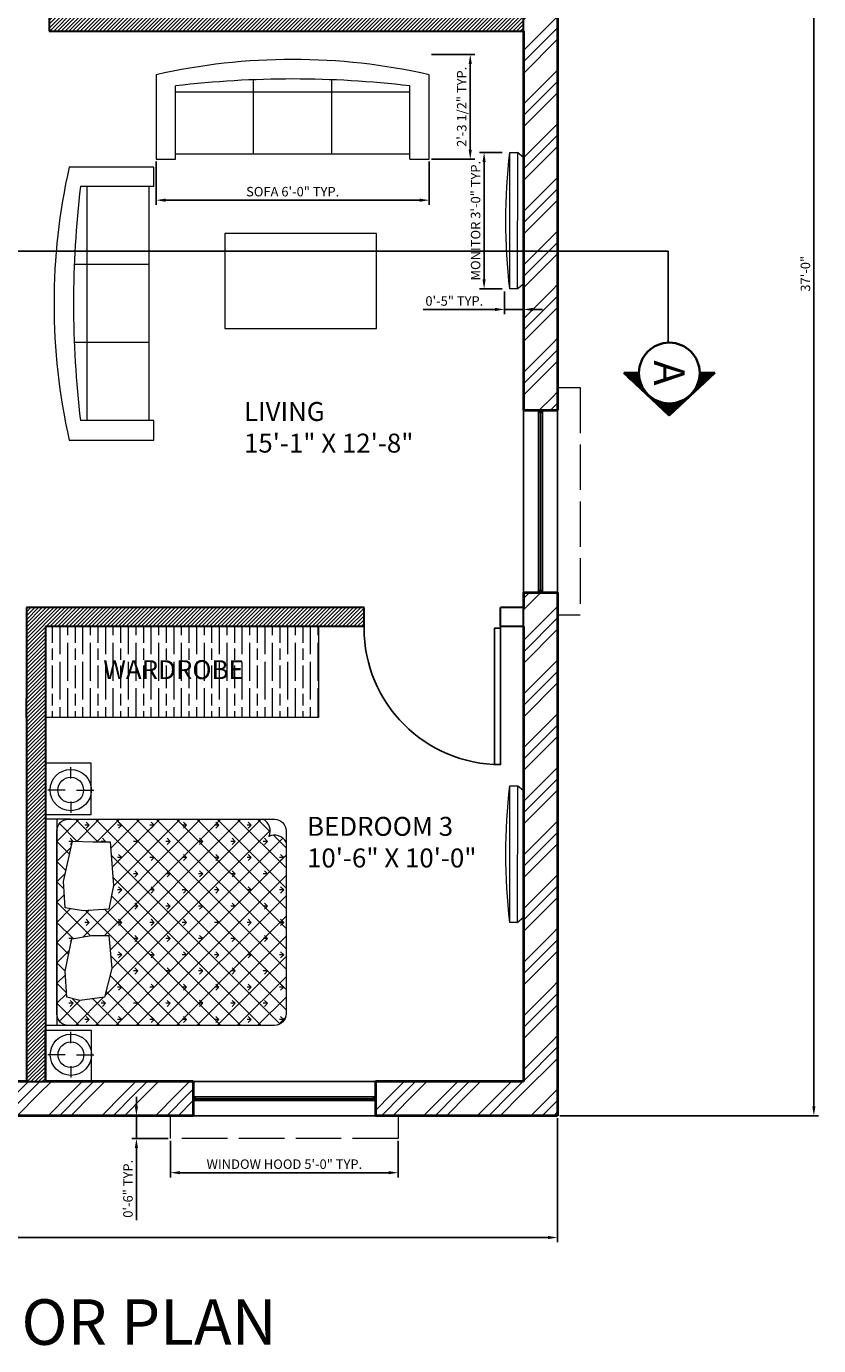
# Model space of a CAD drawing. Units: inches. Extents: x 2443635 to 2446153, y 1826255 to 1827341.
# Tile 4 of 16: x 2443891 to 2444100, y 1826801 to 1827149. Entities that reach past the tile are written whole.
import ezdxf
from ezdxf.enums import TextEntityAlignment as Align

# ---------------------------------------------------------------- set-up
doc = ezdxf.new("R2010")
doc.units = ezdxf.units.IN
doc.linetypes.add('ACAD_ISO02W100', pattern=[15, 12, -3])
for name, color, linetype, lineweight in [('A-ANNO-SYMB', 4, 'Continuous', 25), ('A-DIMS', 1, 'Continuous', 18), ('A-DOOR', 2, 'Continuous', 25), ('A-EQPM', 8, 'Continuous', 18), ('A-FLOR-CASE', 8, 'Continuous', 18), ('A-FLOR-CASE-PATT', 252, 'Continuous', 13), ('A-FURN', 6, 'Continuous', 18), ('A-ROOM', 4, 'Continuous', 18), ('A-SECT', 7, 'Continuous', 35), ('A-TEXT', 4, 'Continuous', 25), ('A-WALL-EXT', 7, 'Continuous', 40), ('A-WALL-INT', 9, 'Continuous', 30), ('A-WALL-OVHD', 7, 'ACAD_ISO02W100', 18), ('A-WALL-PATT', 8, 'Continuous', 13), ('A-WINDOW', 4, 'Continuous', 25)]:
    doc.layers.add(name, color=color, linetype=linetype, lineweight=lineweight)
doc.styles.add('KH-TRUC', font='txt', dxfattribs={"height": 200})
doc.styles.get("Standard").update_dxf_attribs({"font": 'arial.ttf'})
doc.dimstyles.new('ISO-25', dxfattribs={"dimtxt": 2.5, "dimasz": 2.5, "dimexe": 1.25, "dimexo": 0.625, "dimtad": 1, "dimlunit": 4, "dimtxsty": 'Standard', "dimcen": 2.5, "dimadec": 0, "dimazin": 0, "dimtfac": 1, "dimtmove": 0, "dimatfit": 3, "dimfxl": 1, "dimarcsym": 0})

# ---------------------------------------------------------------- blocks, each defined once
blk = doc.blocks.new('*U3')
for p, q in [((0, 0), (0, -6)), ((-40, 0), (-40, -6))]:
    blk.add_line(p, q)
blk.add_lwpolyline([(0, 0), (0, 40), (-1.75, 40), (-1.75, 0)], close=True)
blk.add_arc((0, 0), 40, 90, 180)
blk = doc.blocks.new('*X6')
at = {"color": 0}
for p, q in [((0, 0), (0, 0)), ((-707, -141), (-734, -115)), ((-707, -141), (-707, -104)), ((-707, -141), (-681, -115)), ((-566, 0), (-566, 0)), ((-566, 0), (-566, 0)), ((-283, 0), (-283, 0)), ((-283, 0), (-283, 0)), ((-156, -126), (-168, -115)), ((-141, -141), (-141, -104)), ((-141, -141), (-115, -115)), ((120, -120), (115, -115)), ((283, 0), (283, 0)), ((566, 0), (566, 0)), ((699, -134), (681, -115)), ((707, -135), (707, -104)), ((710, -139), (734, -115)), ((-141, -141), (-142, -140)), ((-849, -283), (-875, -256)), ((-849, -283), (-849, -245)), ((-849, -283), (-822, -256)), ((0, -283), (-27, -256)), ((0, -283), (0, -245)), ((0, -283), (27, -256)), ((849, -283), (822, -256)), ((849, -283), (849, -245)), ((849, -283), (875, -256)), ((-707, -424), (-734, -398)), ((-707, -424), (-707, -387)), ((-707, -424), (-681, -398)), ((-116, -399), (-115, -398)), ((707, -424), (703, -420)), ((707, -424), (707, -387)), ((707, -424), (734, -398)), ((-849, -566), (-875, -539)), ((-849, -566), (-849, -528)), ((-849, -566), (-822, -539)), ((-566, -566), (-592, -539)), ((-566, -566), (-566, -528)), ((-566, -566), (-539, -539)), ((-283, -566), (-309, -539)), ((-283, -566), (-283, -528)), ((-283, -566), (-256, -539)), ((0, -566), (-27, -539)), ((0, -566), (0, -528)), ((0, -566), (27, -539)), ((283, -566), (256, -539)), ((283, -566), (283, -528)), ((283, -566), (309, -539)), ((566, -566), (539, -539)), ((566, -566), (566, -528)), ((566, -566), (592, -539)), ((849, -566), (822, -539)), ((849, -566), (849, -528)), ((849, -566), (875, -539)), ((-707, -707), (-734, -681)), ((-707, -707), (-707, -670)), ((-707, -707), (-681, -681)), ((-424, -707), (-451, -681)), ((-424, -707), (-424, -670)), ((-424, -707), (-398, -681)), ((-141, -707), (-168, -681)), ((-141, -707), (-141, -670)), ((-141, -707), (-115, -681)), ((141, -707), (115, -681)), ((141, -707), (141, -670)), ((141, -707), (168, -681)), ((424, -707), (398, -681)), ((424, -707), (424, -670)), ((424, -707), (451, -681)), ((707, -707), (681, -681)), ((707, -707), (707, -670)), ((707, -707), (734, -681)), ((-849, -849), (-875, -822)), ((-849, -849), (-849, -811)), ((-849, -849), (-822, -822)), ((-566, -849), (-592, -822)), ((-566, -849), (-566, -811)), ((-566, -849), (-539, -822)), ((-283, -849), (-309, -822)), ((-283, -849), (-283, -811)), ((-283, -849), (-256, -822)), ((0, -849), (-27, -822)), ((0, -849), (0, -811)), ((0, -849), (27, -822)), ((283, -849), (256, -822)), ((283, -849), (283, -811)), ((283, -849), (309, -822)), ((566, -849), (539, -822)), ((566, -849), (566, -811)), ((566, -849), (592, -822)), ((849, -849), (822, -822)), ((849, -849), (849, -811)), ((849, -849), (875, -822)), ((-707, -990), (-734, -963)), ((-707, -990), (-707, -952)), ((-707, -990), (-681, -963)), ((-424, -990), (-451, -963)), ((-424, -990), (-424, -952)), ((-424, -990), (-398, -963)), ((-141, -990), (-168, -963)), ((-141, -990), (-141, -952)), ((-141, -990), (-115, -963)), ((141, -990), (115, -963)), ((141, -990), (141, -952)), ((141, -990), (168, -963)), ((424, -990), (398, -963)), ((424, -990), (424, -952)), ((424, -990), (451, -963)), ((707, -990), (681, -963)), ((707, -990), (707, -952)), ((707, -990), (734, -963)), ((-849, -1131), (-875, -1105)), ((-849, -1131), (-849, -1094)), ((-849, -1131), (-822, -1105)), ((-566, -1131), (-592, -1105)), ((-566, -1131), (-566, -1094)), ((-566, -1131), (-539, -1105)), ((-283, -1131), (-309, -1105)), ((-283, -1131), (-283, -1094)), ((-283, -1131), (-256, -1105)), ((0, -1131), (-27, -1105)), ((0, -1131), (0, -1094)), ((0, -1131), (27, -1105)), ((283, -1131), (256, -1105)), ((283, -1131), (283, -1094)), ((283, -1131), (309, -1105)), ((566, -1131), (539, -1105)), ((566, -1131), (566, -1094)), ((566, -1131), (592, -1105)), ((849, -1131), (822, -1105)), ((849, -1131), (849, -1094)), ((849, -1131), (875, -1105)), ((-707, -1273), (-734, -1246)), ((-707, -1273), (-707, -1235)), ((-707, -1273), (-681, -1246)), ((-424, -1273), (-451, -1246)), ((-424, -1273), (-424, -1235)), ((-424, -1273), (-398, -1246)), ((-141, -1273), (-168, -1246)), ((-141, -1273), (-141, -1235)), ((-141, -1273), (-115, -1246)), ((141, -1273), (115, -1246)), ((141, -1273), (141, -1235)), ((141, -1273), (168, -1246)), ((424, -1273), (398, -1246)), ((424, -1273), (424, -1235)), ((424, -1273), (451, -1246)), ((707, -1273), (681, -1246)), ((707, -1273), (707, -1235)), ((707, -1273), (734, -1246)), ((-849, -1414), (-849, -1377)), ((-566, -1414), (-566, -1377)), ((-283, -1414), (-283, -1377)), ((0, -1414), (0, -1377)), ((283, -1414), (283, -1377)), ((566, -1414), (566, -1377)), ((849, -1414), (849, -1377)), ((-849, -1414), (-875, -1388)), ((-849, -1414), (-822, -1388)), ((-566, -1414), (-592, -1388)), ((-566, -1414), (-539, -1388)), ((-283, -1414), (-309, -1388)), ((-283, -1414), (-256, -1388)), ((0, -1414), (-27, -1388)), ((0, -1414), (27, -1388)), ((283, -1414), (256, -1388)), ((283, -1414), (309, -1388)), ((566, -1414), (539, -1388)), ((566, -1414), (592, -1388)), ((849, -1414), (822, -1388)), ((849, -1414), (875, -1388)), ((-707, -1556), (-734, -1529)), ((-707, -1556), (-707, -1518)), ((-707, -1556), (-681, -1529)), ((-424, -1556), (-451, -1529)), ((-424, -1556), (-424, -1518)), ((-424, -1556), (-398, -1529)), ((-141, -1556), (-168, -1529)), ((-141, -1556), (-141, -1518)), ((-141, -1556), (-115, -1529)), ((141, -1556), (115, -1529)), ((141, -1556), (141, -1518)), ((141, -1556), (168, -1529)), ((424, -1556), (398, -1529)), ((424, -1556), (424, -1518)), ((424, -1556), (451, -1529)), ((707, -1556), (681, -1529)), ((707, -1556), (707, -1518)), ((707, -1556), (734, -1529)), ((-849, -1697), (-875, -1671)), ((-849, -1697), (-849, -1660)), ((-849, -1697), (-822, -1671)), ((-566, -1697), (-592, -1671)), ((-566, -1697), (-566, -1660)), ((-566, -1697), (-539, -1671)), ((-283, -1697), (-309, -1671)), ((-283, -1697), (-283, -1660)), ((-283, -1697), (-256, -1671)), ((0, -1697), (-27, -1671)), ((0, -1697), (0, -1660)), ((0, -1697), (27, -1671)), ((283, -1697), (256, -1671)), ((283, -1697), (283, -1660)), ((283, -1697), (309, -1671)), ((566, -1697), (539, -1671)), ((566, -1697), (566, -1660)), ((566, -1697), (592, -1671)), ((849, -1697), (822, -1671)), ((849, -1697), (849, -1660)), ((849, -1697), (875, -1671)), ((-707, -1838), (-734, -1812)), ((-707, -1838), (-707, -1801)), ((-707, -1838), (-681, -1812)), ((-424, -1838), (-451, -1812)), ((-424, -1838), (-424, -1801)), ((-424, -1838), (-398, -1812)), ((-141, -1838), (-168, -1812)), ((-141, -1838), (-141, -1801)), ((-141, -1838), (-115, -1812)), ((141, -1838), (115, -1812)), ((141, -1838), (141, -1801)), ((141, -1838), (168, -1812)), ((424, -1838), (398, -1812)), ((424, -1838), (424, -1801)), ((424, -1838), (451, -1812)), ((707, -1838), (681, -1812)), ((707, -1838), (707, -1801)), ((707, -1838), (734, -1812)), ((-849, -1980), (-875, -1953)), ((-849, -1980), (-849, -1942)), ((-849, -1980), (-822, -1953)), ((-566, -1980), (-592, -1953)), ((-566, -1980), (-566, -1942)), ((-566, -1980), (-539, -1953)), ((-283, -1980), (-309, -1953)), ((-283, -1980), (-283, -1942)), ((-283, -1980), (-256, -1953)), ((0, -1980), (-27, -1953)), ((0, -1980), (0, -1942)), ((0, -1980), (27, -1953)), ((283, -1980), (256, -1953)), ((283, -1980), (283, -1942)), ((283, -1980), (309, -1953)), ((566, -1980), (539, -1953)), ((566, -1980), (566, -1942)), ((566, -1980), (592, -1953))]:
    blk.add_line(p, q, dxfattribs=at)
blk = doc.blocks.new('*X5')
at = {"color": 0}
for p, q in [((-900, -193), (-707, 0)), ((-623, -84), (-707, 0)), ((-614, -83), (-530, 0)), ((-457, -74), (-530, 0)), ((-425, -72), (-354, 0)), ((-245, -108), (-354, 0)), ((-278, -101), (-177, 0)), ((103, -280), (-177, 0)), ((-142, -142), (0, 0)), ((-117, -294), (177, 0)), ((120, -120), (0, 0)), ((241, -64), (177, 0)), ((292, -61), (354, 0)), ((426, -72), (354, 0)), ((452, -78), (530, 0)), ((654, -123), (530, 0)), ((596, -111), (707, 0)), ((900, -193), (707, 0)), ((-683, -201), (-862, -22)), ((708, -175), (862, -22)), ((-900, -370), (-667, -137)), ((-656, -405), (-900, -161)), ((900, -1254), (-128, -225)), ((703, -358), (900, -161)), ((900, -370), (708, -178)), ((-900, -1254), (101, -252)), ((-900, -546), (-668, -314)), ((735, -1973), (-900, -337)), ((-763, -2000), (900, -337)), ((-900, -1430), (112, -418)), ((-900, -723), (-605, -429)), ((801, -1862), (-641, -419)), ((900, -1430), (-116, -415)), ((900, -546), (703, -349)), ((-900, -900), (-465, -465)), ((-900, -1077), (-293, -470)), ((-900, -1607), (231, -476)), ((-900, -1784), (394, -489)), ((586, -2000), (-900, -514)), ((-888, -1948), (586, -475)), ((-586, -2000), (900, -514)), ((900, -1784), (-404, -480)), ((900, -1607), (-243, -465)), ((900, -1077), (317, -494)), ((900, -900), (483, -483)), ((900, -723), (647, -470)), ((409, -2000), (-900, -691)), ((-409, -2000), (900, -691)), ((232, -2000), (-900, -868)), ((-232, -2000), (900, -868)), ((55, -2000), (-900, -1045)), ((-55, -2000), (900, -1045)), ((-121, -2000), (-900, -1221)), ((121, -2000), (900, -1221)), ((-298, -2000), (-900, -1398)), ((298, -2000), (900, -1398)), ((-475, -2000), (-900, -1575)), ((475, -2000), (900, -1575)), ((-652, -2000), (-900, -1752)), ((790, -1861), (900, -1752)), ((-835, -1994), (-894, -1935)), ((652, -2000), (761, -1890))]:
    blk.add_line(p, q, dxfattribs=at)
blk = doc.blocks.new('A$C190D2546')
at = {"layer": 'A-FURN'}
for p, q in [((285, 1928), (285, 2078)), ((541, 2100), (2341, 2100)), ((541, 1881), (541, 2100)), ((2341, 1881), (2341, 2100)), ((2596, 1929), (2596, 2079)), ((2341, 2000), (541, 2000)), ((185, 1878), (85, 1878)), ((385, 1878), (485, 1878)), ((2496, 1879), (2396, 1879)), ((2696, 1879), (2796, 1879)), ((285, 1828), (285, 1678)), ((2596, 1829), (2596, 1679))]:
    blk.add_line(p, q, dxfattribs=at)
for points in [[(500, 2101), (500, 1701), (50, 1701), (50, 2101)], [(2382, 2101), (2382, 1701), (2832, 1701), (2832, 2101)], [(787, 1584), (758, 1799), (787, 1914), (1016, 1928), (1296, 1871), (1325, 1699), (1325, 1548), (1038, 1519)], [(1555, 1548), (1541, 1771), (1569, 1928), (1799, 1943), (2151, 1864), (2144, 1685), (2144, 1534), (1763, 1505)]]:
    blk.add_lwpolyline(points, close=True, dxfattribs=at)
blk.add_lwpolyline([(641, 2000), (2241, 2000, -0.414214), (2341, 1900), (2341, 100, -0.414214), (2241, 0), (641, 0, -0.414214), (541, 100), (541, 1900, -0.414214)], format="xyb", close=True, dxfattribs=at)
for centre, radius in [((285, 1878), 180), ((285, 1878), 112), ((2596, 1879), 180), ((2596, 1879), 112)]:
    blk.add_circle(centre, radius, dxfattribs=at)
for centre, start, end in [((2091, 100), 296.5651, 26.5651), ((2241, 250), 243.4349, 333.4349)]:
    blk.add_arc(centre, 112, start, end, dxfattribs=at)
for name in ['*X5', '*X6']:
    blk.add_blockref(name, (1441, 2000), dxfattribs=at)
blk = doc.blocks.new('LCD Monitor Pln')
at = {"layer": 'A-FURN'}
for p, q in [((5656.37, -10564.55), (5660.02, -10561.47)), ((5656.37, -10564.55), (5656.4, -10641.11)), ((5660.02, -10561.47), (5660.05, -10644.19)), ((5664.53, -10561.47), (5660.02, -10561.47)), ((5664.56, -10644.19), (5664.53, -10561.47)), ((5660.05, -10644.19), (5656.4, -10641.11)), ((5660.05, -10644.19), (5664.56, -10644.19))]:
    blk.add_line(p, q, dxfattribs=at)
blk.add_arc((5310.21, -10602.95), 356.75, 353.36301, 6.67799, dxfattribs=at)
blk = doc.blocks.new('*X15')
at = {"color": 0}
for p, q in [((19.68, 20.47), (19.71, 20.51)), ((19.68, 20.38), (19.76, 20.46)), ((19.68, 20.29), (19.8, 20.42)), ((19.68, 20.21), (19.84, 20.37)), ((19.68, 20.12), (19.88, 20.33)), ((19.68, 20.03), (19.93, 20.28)), ((19.68, 19.94), (19.97, 20.23)), ((19.68, 19.85), (20.01, 20.19)), ((19.68, 19.76), (20.05, 20.14)), ((19.68, 19.68), (20.1, 20.1)), ((19.68, 19.59), (20.14, 20.05)), ((19.68, 19.5), (20.18, 20.01)), ((19.68, 19.41), (20.22, 19.96)), ((19.68, 19.32), (20.27, 19.91)), ((19.68, 19.23), (20.31, 19.87)), ((19.68, 19.15), (20.35, 19.82)), ((19.68, 19.06), (20.4, 19.78)), ((19.68, 18.97), (20.44, 19.73)), ((19.68, 18.88), (20.48, 19.69)), ((19.68, 18.79), (20.52, 19.64)), ((19.68, 18.7), (20.57, 19.59)), ((19.68, 18.62), (20.61, 19.55)), ((19.68, 18.53), (20.65, 19.5)), ((19.68, 18.44), (20.69, 19.46)), ((19.68, 18.35), (20.74, 19.41)), ((19.68, 18.26), (20.78, 19.37)), ((19.68, 18.17), (20.82, 19.32)), ((19.68, 18.08), (20.86, 19.27)), ((19.73, 18.05), (20.91, 19.23)), ((19.81, 18.05), (20.95, 19.18)), ((19.9, 18.04), (20.99, 19.14)), ((19.98, 18.04), (21.04, 19.09)), ((20.06, 18.03), (21.08, 19.05)), ((20.15, 18.03), (21.12, 19)), ((20.23, 18.02), (21.16, 18.95)), ((20.31, 18.01), (21.21, 18.91)), ((20.38, 18), (21.25, 18.86)), ((20.46, 17.99), (21.29, 18.82)), ((20.54, 17.97), (21.33, 18.77)), ((20.61, 17.96), (21.38, 18.73)), ((20.68, 17.94), (21.42, 18.68)), ((20.76, 17.93), (21.46, 18.63)), ((20.83, 17.91), (21.5, 18.59)), ((20.9, 17.9), (21.55, 18.54)), ((20.97, 17.88), (21.59, 18.5)), ((21.04, 17.86), (21.63, 18.45)), ((21.11, 17.84), (21.68, 18.41)), ((21.18, 17.82), (21.72, 18.36)), ((21.24, 17.8), (21.76, 18.31)), ((21.31, 17.77), (21.8, 18.27)), ((21.37, 17.75), (21.85, 18.22)), ((21.44, 17.73), (21.89, 18.18)), ((21.5, 17.7), (21.93, 18.13)), ((21.57, 17.68), (21.97, 18.08)), ((21.63, 17.65), (22.02, 18.04)), ((21.69, 17.62), (22.06, 17.99)), ((21.75, 17.6), (22.1, 17.95)), ((21.81, 17.57), (22.14, 17.9)), ((21.87, 17.54), (22.19, 17.86)), ((21.93, 17.51), (22.23, 17.81)), ((21.99, 17.48), (22.27, 17.76)), ((22.05, 17.45), (22.32, 17.72)), ((22.1, 17.42), (22.36, 17.67)), ((22.16, 17.39), (22.4, 17.63)), ((22.22, 17.35), (22.44, 17.58)), ((22.27, 17.32), (22.49, 17.54)), ((22.33, 17.29), (22.53, 17.49)), ((22.38, 17.25), (22.57, 17.44)), ((22.43, 17.22), (22.61, 17.4)), ((22.49, 17.18), (22.66, 17.35)), ((22.54, 17.15), (22.7, 17.31)), ((22.59, 17.11), (22.74, 17.26)), ((22.64, 17.07), (22.78, 17.22)), ((22.69, 17.04), (22.83, 17.17)), ((22.74, 17), (22.87, 17.12)), ((22.79, 16.96), (22.91, 17.08)), ((22.84, 16.92), (22.96, 17.03)), ((22.89, 16.88), (23, 16.99)), ((22.94, 16.84), (23.04, 16.94)), ((22.98, 16.8), (23.08, 16.9)), ((23.03, 16.75), (23.13, 16.85)), ((23.08, 16.71), (23.17, 16.8)), ((23.12, 16.67), (23.21, 16.76)), ((23.17, 16.63), (23.25, 16.71)), ((23.21, 16.58), (23.3, 16.67)), ((23.26, 16.54), (23.34, 16.62)), ((23.3, 16.49), (23.38, 16.58)), ((23.34, 16.45), (23.42, 16.53)), ((23.38, 16.4), (23.47, 16.48)), ((23.43, 16.35), (23.51, 16.44)), ((23.47, 16.31), (23.55, 16.39)), ((23.51, 16.26), (23.6, 16.35)), ((23.55, 16.21), (23.64, 16.3)), ((23.59, 16.16), (23.68, 16.26)), ((23.63, 16.11), (23.72, 16.21)), ((23.66, 16.06), (23.77, 16.16)), ((23.7, 16.01), (23.81, 16.12)), ((23.74, 15.96), (23.85, 16.07)), ((23.78, 15.91), (23.89, 16.03)), ((23.81, 15.86), (23.94, 15.98)), ((23.85, 15.8), (23.98, 15.94)), ((23.88, 15.75), (24.02, 15.89)), ((23.92, 15.7), (24.06, 15.84)), ((23.95, 15.64), (24.11, 15.8)), ((23.98, 15.59), (24.15, 15.75)), ((24.02, 15.53), (24.19, 15.71)), ((24.05, 15.47), (24.24, 15.66)), ((24.08, 15.42), (24.28, 15.62)), ((24.11, 15.36), (24.32, 15.57)), ((24.14, 15.3), (24.36, 15.52)), ((24.17, 15.24), (24.41, 15.48)), ((24.2, 15.18), (24.45, 15.43)), ((24.23, 15.12), (24.49, 15.39)), ((24.25, 15.06), (24.53, 15.34)), ((24.28, 15), (24.58, 15.3)), ((24.31, 14.94), (24.62, 15.25)), ((23.72, 10.11), (26.67, 13.06)), ((23.91, 10.38), (26.63, 13.1)), ((24.04, 10.6), (26.58, 13.15)), ((24.14, 10.79), (26.54, 13.19)), ((24.22, 10.96), (26.5, 13.24)), ((24.29, 11.12), (26.45, 13.28)), ((24.33, 14.87), (24.66, 15.2)), ((24.35, 11.27), (26.41, 13.33)), ((24.36, 14.81), (24.7, 15.16)), ((24.38, 14.74), (24.75, 15.11)), ((24.4, 14.68), (24.79, 15.07)), ((24.4, 11.41), (26.37, 13.38)), ((24.42, 14.61), (24.83, 15.02)), ((24.44, 11.54), (26.33, 13.42)), ((24.45, 14.55), (24.88, 14.98)), ((24.47, 14.48), (24.92, 14.93)), ((24.48, 11.66), (26.28, 13.47)), ((24.49, 14.41), (24.96, 14.88)), ((24.51, 14.34), (25, 14.84)), ((24.51, 11.79), (26.24, 13.51)), ((24.52, 14.27), (25.05, 14.79)), ((24.54, 14.2), (25.09, 14.75)), ((24.54, 11.9), (26.2, 13.56)), ((24.56, 14.13), (25.13, 14.7)), ((24.57, 14.06), (25.17, 14.66)), ((24.57, 12.02), (26.16, 13.6)), ((24.59, 13.98), (25.22, 14.61)), ((24.59, 12.13), (26.11, 13.65)), ((24.6, 13.91), (25.26, 14.56)), ((24.61, 13.83), (25.3, 14.52)), ((24.61, 12.24), (26.07, 13.7)), ((24.63, 13.75), (25.35, 14.47)), ((24.63, 12.34), (26.03, 13.74)), ((24.64, 13.68), (25.39, 14.43)), ((24.64, 12.44), (25.99, 13.79)), ((24.65, 13.6), (25.43, 14.38)), ((24.65, 13.52), (25.47, 14.34)), ((24.65, 12.54), (25.94, 13.83)), ((24.66, 13.44), (25.52, 14.29)), ((24.66, 12.64), (25.9, 13.88)), ((24.67, 13.35), (25.56, 14.24)), ((24.67, 13.27), (25.6, 14.2)), ((24.67, 13.18), (25.64, 14.15)), ((24.67, 12.92), (25.77, 14.02)), ((24.67, 12.83), (25.81, 13.97)), ((24.67, 12.73), (25.86, 13.92)), ((24.68, 13.1), (25.69, 14.11)), ((24.68, 13.01), (25.73, 14.06)), ((19.68, 5.98), (25.68, 11.98)), ((19.68, 5.89), (24.44, 10.65)), ((19.68, 5.8), (23.2, 9.32)), ((19.68, 6.06), (22.61, 9)), ((19.68, 6.15), (22.34, 8.81)), ((19.68, 6.24), (22.12, 8.69)), ((19.68, 6.33), (21.93, 8.58)), ((19.68, 6.42), (21.76, 8.5)), ((19.68, 6.51), (21.6, 8.43)), ((19.68, 6.59), (21.46, 8.37)), ((19.68, 6.68), (21.32, 8.32)), ((19.68, 6.77), (21.19, 8.28)), ((19.68, 6.86), (21.06, 8.24)), ((19.68, 6.95), (20.94, 8.21)), ((19.68, 7.04), (20.82, 8.18)), ((19.68, 7.12), (20.71, 8.15)), ((19.68, 7.21), (20.6, 8.13)), ((19.68, 7.3), (20.49, 8.11)), ((19.68, 7.39), (20.38, 8.1)), ((19.68, 7.48), (20.28, 8.08)), ((19.68, 7.57), (20.18, 8.07)), ((19.68, 7.74), (19.99, 8.06)), ((19.68, 7.66), (20.08, 8.06)), ((19.68, 8.01), (19.71, 8.05)), ((19.68, 7.92), (19.8, 8.05)), ((19.68, 7.83), (19.9, 8.05)), ((19.68, 5.71), (21.96, 8)), ((19.68, 5.62), (20.73, 6.67))]:
    blk.add_line(p, q, dxfattribs=at)
blk = doc.blocks.new('A$C0BB45C51')
at = {"layer": 'A-SECT'}
for p, q in [((12.86, 15), (19.86, 7.5)), ((12.86, 12.5), (12.86, 15)), ((12.86, 0), (19.86, 7.5)), ((12.86, 2.5), (12.86, 0))]:
    blk.add_line(p, q, dxfattribs=at)
blk.add_circle((12.86, 7.5), 5, dxfattribs=at)
blk.add_blockref('*X15', (-6.82, -5.55), dxfattribs=at)
at = {"layer": 'A-SECT', "style": 'KH-TRUC'}
blk.add_attdef('KH-MC', text='', height=5, dxfattribs=at).set_placement((12.86, 7.5), align=Align.MIDDLE_CENTER)
blk = doc.blocks.new('SOFA-3-SEAT')
at = {"transparency": 33554687}
for p, q in [((0, 22.29), (0, 0)), ((25.71, 1.34), (25.71, 20.94)), ((46.29, 1.34), (46.29, 20.94)), ((72, 0), (72, 22.29)), ((5.14, 0), (5.14, 19.31)), ((66.86, 17.67), (5.14, 17.67)), ((66.86, 0), (66.86, 19.31)), ((0, 0), (5.14, 0)), ((66.86, 1.34), (5.14, 1.34)), ((66.86, 0), (72, 0))]:
    blk.add_line(p, q, dxfattribs=at)
for centre, radius, start, end in [((36, -137.71), 164, 77.3196, 102.6804), ((36, -239.71), 260.86, 83.2065, 96.7935)]:
    blk.add_arc(centre, radius, start, end, dxfattribs=at)
blk = doc.blocks.new('COFFEE-TABLE-40X25')
at = {"transparency": 33554687}
for p, q in [((0, 25), (0, 0)), ((40, 25), (0, 25)), ((40, 0), (40, 25)), ((0, 0), (40, 0))]:
    blk.add_line(p, q, dxfattribs=at)
blk = doc.blocks.new('WIN-48-PLAN')
at = {"transparency": 33554687}
for p, q in [((0, 0), (0, 48)), ((0, 48), (9, 48)), ((4, 48), (4, 0)), ((4, 47.5), (5, 47.5)), ((4.5, 47.5), (4.5, 0.5)), ((5, 48), (5, 0)), ((9, 48), (9, 0)), ((5, 0.5), (4, 0.5)), ((9, 0), (0, 0))]:
    blk.add_line(p, q, dxfattribs=at)
blk = doc.blocks.new('WINDOW-HOOD-60-PLAN')
at = {"transparency": 33554687}
for p, q in [((0, 60), (6, 60)), ((6, 60), (6, 0)), ((6, 0), (0, 0))]:
    blk.add_line(p, q, dxfattribs=at)
blk = doc.blocks.new('*D54')
at = {"layer": 'A-DIMS', "color": 0, "lineweight": -2, "transparency": 16777216}
for p, q in [((2443925.28, 1827112.87), (2443925.28, 1827101.45)), ((2443997.28, 1827112.87), (2443997.28, 1827101.45)), ((2443927.78, 1827102.7), (2443994.78, 1827102.7))]:
    blk.add_line(p, q, dxfattribs=at)
at = {"layer": 'A-DIMS', "color": 0, "transparency": 16777216}
for points in [[(2443927.78, 1827103.11), (2443927.78, 1827102.28), (2443925.28, 1827102.7)], [(2443994.78, 1827103.11), (2443994.78, 1827102.28), (2443997.28, 1827102.7)]]:
    blk.add_solid(points, dxfattribs=at)
at = {"layer": 'Defpoints', "color": 0, "transparency": 16777216}
for p in [(2443925.28, 1827113.5), (2443997.28, 1827113.5), (2443997.28, 1827102.7)]:
    blk.add_point(p, dxfattribs=at)
at = {"layer": 'A-DIMS', "color": 0, "transparency": 16777216, "insert": (2443961.28, 1827104.62), "char_height": 2.5, "attachment_point": 5}
blk.add_mtext('SOFA 6\'-0" TYP.', dxfattribs=at)
blk = doc.blocks.new('*D55')
at = {"layer": 'A-DIMS', "color": 0, "lineweight": -2, "transparency": 16777216}
for p, q in [((2443997.91, 1827141.12), (2444009.33, 1827141.12)), ((2444008.08, 1827116), (2444008.08, 1827138.62)), ((2443997.91, 1827113.5), (2444009.33, 1827113.5))]:
    blk.add_line(p, q, dxfattribs=at)
at = {"layer": 'A-DIMS', "color": 0, "transparency": 16777216}
for points in [[(2444007.67, 1827138.62), (2444008.5, 1827138.62), (2444008.08, 1827141.12)], [(2444007.67, 1827116), (2444008.5, 1827116), (2444008.08, 1827113.5)]]:
    blk.add_solid(points, dxfattribs=at)
at = {"layer": 'Defpoints', "color": 0, "transparency": 16777216}
for p in [(2443997.28, 1827141.12), (2444008.08, 1827141.12), (2443997.28, 1827113.5)]:
    blk.add_point(p, dxfattribs=at)
at = {"layer": 'A-DIMS', "color": 0, "transparency": 16777216, "insert": (2444006.16, 1827127.31), "char_height": 2.5, "attachment_point": 5, "rotation": 90}
blk.add_mtext('2\'-3 1/2" TYP.', dxfattribs=at)
blk = doc.blocks.new('*D62')
at = {"layer": 'A-DIMS', "color": 0, "lineweight": -2, "transparency": 16777216}
for p, q in [((2444016.51, 1827115.29), (2444010.49, 1827115.29)), ((2444011.74, 1827081.79), (2444011.74, 1827112.79)), ((2444016.51, 1827079.29), (2444010.49, 1827079.29))]:
    blk.add_line(p, q, dxfattribs=at)
at = {"layer": 'A-DIMS', "color": 0, "transparency": 16777216}
for points in [[(2444011.32, 1827112.79), (2444012.15, 1827112.79), (2444011.74, 1827115.29)], [(2444011.32, 1827081.79), (2444012.15, 1827081.79), (2444011.74, 1827079.29)]]:
    blk.add_solid(points, dxfattribs=at)
at = {"layer": 'Defpoints', "color": 0, "transparency": 16777216}
for p in [(2444011.74, 1827115.29), (2444017.14, 1827115.29), (2444017.14, 1827079.29)]:
    blk.add_point(p, dxfattribs=at)
at = {"layer": 'A-DIMS', "color": 0, "transparency": 16777216, "insert": (2444009.82, 1827097.29), "char_height": 2.5, "attachment_point": 5, "rotation": 90}
blk.add_mtext('MONITOR 3\'-0" TYP.', dxfattribs=at)
blk = doc.blocks.new('*D63')
at = {"layer": 'A-DIMS', "color": 0, "lineweight": -2, "transparency": 16777216}
for p, q in [((2444017.14, 1827078.66), (2444017.14, 1827072.64)), ((2444022.1, 1827078.66), (2444022.1, 1827072.64)), ((2444014.64, 1827073.89), (2443995.65, 1827073.89)), ((2444022.1, 1827073.89), (2444017.14, 1827073.89)), ((2444024.6, 1827073.89), (2444027.1, 1827073.89))]:
    blk.add_line(p, q, dxfattribs=at)
at = {"layer": 'A-DIMS', "color": 0, "transparency": 16777216}
for points in [[(2444014.64, 1827074.31), (2444014.64, 1827073.47), (2444017.14, 1827073.89)], [(2444024.6, 1827074.31), (2444024.6, 1827073.47), (2444022.1, 1827073.89)]]:
    blk.add_solid(points, dxfattribs=at)
at = {"layer": 'Defpoints', "color": 0, "transparency": 16777216}
for p in [(2444017.14, 1827079.29), (2444022.1, 1827079.29), (2444017.14, 1827073.89)]:
    blk.add_point(p, dxfattribs=at)
at = {"layer": 'A-DIMS', "color": 0, "transparency": 16777216, "insert": (2444003.89, 1827075.79), "char_height": 2.5, "attachment_point": 5}
blk.add_mtext('0\'-5" TYP.', dxfattribs=at)
blk = doc.blocks.new('*D66')
at = {"layer": 'A-DIMS', "color": 0, "lineweight": -2, "transparency": 16777216}
for p, q in [((2443929.09, 1826854.66), (2443929.09, 1826845.04)), ((2443989.09, 1826854.66), (2443989.09, 1826845.04)), ((2443931.59, 1826846.29), (2443986.59, 1826846.29))]:
    blk.add_line(p, q, dxfattribs=at)
at = {"layer": 'A-DIMS', "color": 0, "transparency": 16777216}
for points in [[(2443931.59, 1826846.7), (2443931.59, 1826845.87), (2443929.09, 1826846.29)], [(2443986.59, 1826846.7), (2443986.59, 1826845.87), (2443989.09, 1826846.29)]]:
    blk.add_solid(points, dxfattribs=at)
at = {"layer": 'Defpoints', "color": 0, "transparency": 16777216}
for p in [(2443929.09, 1826855.29), (2443989.09, 1826855.29), (2443989.09, 1826846.29)]:
    blk.add_point(p, dxfattribs=at)
at = {"layer": 'A-DIMS', "color": 0, "transparency": 16777216, "insert": (2443959.09, 1826848.21), "char_height": 2.5, "attachment_point": 5}
blk.add_mtext('WINDOW HOOD 5\'-0" TYP.', dxfattribs=at)
blk = doc.blocks.new('*D67')
at = {"layer": 'A-DIMS', "color": 0, "lineweight": -2, "transparency": 16777216}
for p, q in [((2443920.09, 1826863.79), (2443920.09, 1826866.29)), ((2443928.46, 1826861.29), (2443918.84, 1826861.29)), ((2443920.09, 1826861.29), (2443920.09, 1826855.29)), ((2443928.46, 1826855.29), (2443918.84, 1826855.29)), ((2443920.09, 1826852.79), (2443920.09, 1826833.8))]:
    blk.add_line(p, q, dxfattribs=at)
at = {"layer": 'A-DIMS', "color": 0, "transparency": 16777216}
for points in [[(2443919.67, 1826863.79), (2443920.51, 1826863.79), (2443920.09, 1826861.29)], [(2443919.67, 1826852.79), (2443920.51, 1826852.79), (2443920.09, 1826855.29)]]:
    blk.add_solid(points, dxfattribs=at)
at = {"layer": 'Defpoints', "color": 0, "transparency": 16777216}
for p in [(2443929.09, 1826861.29), (2443920.09, 1826855.29), (2443929.09, 1826855.29)]:
    blk.add_point(p, dxfattribs=at)
at = {"layer": 'A-DIMS', "color": 0, "transparency": 16777216, "insert": (2443918.19, 1826842.04), "char_height": 2.5, "attachment_point": 5, "rotation": 90}
blk.add_mtext('0\'-6" TYP.', dxfattribs=at)
blk = doc.blocks.new('*D90')
at = {"layer": 'A-DIMS', "color": 0, "lineweight": -2, "transparency": 16777216}
for p, q in [((2443707.09, 1826860.66), (2443707.09, 1826827.94)), ((2444031.09, 1826860.66), (2444031.09, 1826827.94)), ((2443709.59, 1826829.19), (2444028.59, 1826829.19))]:
    blk.add_line(p, q, dxfattribs=at)
at = {"layer": 'A-DIMS', "color": 0, "transparency": 16777216}
for points in [[(2443709.59, 1826829.6), (2443709.59, 1826828.77), (2443707.09, 1826829.19)], [(2444028.59, 1826829.6), (2444028.59, 1826828.77), (2444031.09, 1826829.19)]]:
    blk.add_solid(points, dxfattribs=at)
at = {"layer": 'Defpoints', "color": 0, "transparency": 16777216}
for p in [(2443707.09, 1826861.29), (2444031.09, 1826861.29), (2444031.09, 1826829.19)]:
    blk.add_point(p, dxfattribs=at)
at = {"layer": 'A-DIMS', "color": 0, "transparency": 16777216, "insert": (2443869.09, 1826831.09), "char_height": 2.5, "attachment_point": 5}
blk.add_mtext('27\'-0"', dxfattribs=at)
blk = doc.blocks.new('*D91')
at = {"layer": 'A-DIMS', "color": 0, "lineweight": -2, "transparency": 16777216}
for p, q in [((2444031.71, 1827305.29), (2444099.91, 1827305.29)), ((2444098.66, 1826863.79), (2444098.66, 1827302.79)), ((2444031.71, 1826861.29), (2444099.91, 1826861.29))]:
    blk.add_line(p, q, dxfattribs=at)
at = {"layer": 'A-DIMS', "color": 0, "transparency": 16777216}
for points in [[(2444098.25, 1827302.79), (2444099.08, 1827302.79), (2444098.66, 1827305.29)], [(2444098.25, 1826863.79), (2444099.08, 1826863.79), (2444098.66, 1826861.29)]]:
    blk.add_solid(points, dxfattribs=at)
at = {"layer": 'Defpoints', "color": 0, "transparency": 16777216}
for p in [(2444031.09, 1827305.29), (2444098.66, 1827305.29), (2444031.09, 1826861.29)]:
    blk.add_point(p, dxfattribs=at)
at = {"layer": 'A-DIMS', "color": 0, "transparency": 16777216, "insert": (2444096.76, 1827083.29), "char_height": 2.5, "attachment_point": 5, "rotation": 90}
blk.add_mtext('37\'-0"', dxfattribs=at)

msp = doc.modelspace()

# ---------------------------------------------------------------- hatches: boundary and pattern name
at = {"layer": 'A-FLOR-CASE-PATT'}
h = msp.add_hatch(dxfattribs=at)
h.set_pattern_fill('GOST_WOOD', color=256)
h.paths.add_polyline_path([(2443968.09, 1826966.288), (2443968.09, 1826990.288), (2443896.09, 1826990.288), (2443896.09, 1826966.288)])
h.paths.add_polyline_path([(2443902.09, 1827224.288), (2443926.09, 1827224.288), (2443926.09, 1827296.288), (2443902.09, 1827296.288)])
h.paths.add_polyline_path([(2443836.09, 1827296.288), (2443812.09, 1827296.288), (2443812.09, 1827224.288), (2443836.09, 1827224.288)])
at = {"layer": 'A-WALL-PATT'}
h = msp.add_hatch(dxfattribs=at)
h.set_pattern_fill('GOST_GROUND', color=256)
h.paths.add_polyline_path([(2443848.09, 1826870.288), (2443841.09, 1826870.288), (2443836.09, 1826870.288), (2443794.09, 1826870.288), (2443794.09, 1826861.288), (2443848.09, 1826861.288)])
h.paths.add_polyline_path([(2443935.09, 1826870.288), (2443896.09, 1826870.288), (2443891.09, 1826870.288), (2443884.09, 1826870.288), (2443884.09, 1826861.288), (2443935.09, 1826861.288)])
h.paths.add_polyline_path([(2444031.09, 1826999.288), (2444022.09, 1826999.288), (2444022.09, 1826995.288), (2444022.09, 1826990.288), (2444022.09, 1826870.288), (2443983.09, 1826870.288), (2443983.09, 1826861.288), (2444031.09, 1826861.288)])
h.paths.add_polyline_path([(2443758.09, 1826870.288), (2443716.09, 1826870.288), (2443716.09, 1826925.457, -0.0618154), (2443716.09, 1826925.788), (2443716.09, 1826948.288), (2443707.09, 1826948.288), (2443707.09, 1826861.288), (2443758.09, 1826861.288)])
h.paths.add_polyline_path([(2443716.09, 1827062.288), (2443716.09, 1827067.288), (2443716.09, 1827147.288), (2443716.09, 1827152.288), (2443716.09, 1827194.288), (2443707.09, 1827194.288), (2443707.09, 1826984.288), (2443716.09, 1826984.288)])
h.paths.add_polyline_path([(2443716.09, 1827296.288), (2443836.09, 1827296.288), (2443841.09, 1827296.288), (2443860.09, 1827296.288), (2443860.09, 1827305.288), (2443707.09, 1827305.288), (2443707.09, 1827254.288), (2443716.09, 1827254.288)])
h.paths.add_polyline_path([(2444031.09, 1827305.288), (2443878.09, 1827305.288), (2443878.09, 1827296.288), (2443881.588, 1827296.288), (2443897.09, 1827296.288), (2443902.09, 1827296.288), (2444022.09, 1827296.288), (2444022.09, 1827284.209), (2444022.09, 1827254.288), (2444031.09, 1827254.288)])
h.paths.add_polyline_path([(2444031.09, 1827194.288), (2444022.09, 1827194.288), (2444022.09, 1827152.288), (2444022.09, 1827147.288), (2444022.09, 1827113.953), (2444022.096, 1827113.948), (2444022.084, 1827080.628), (2444022.09, 1827047.288), (2444031.09, 1827047.288)])
h = msp.add_hatch(dxfattribs=at)
h.set_pattern_fill('JIS_WOOD', color=256)
h.paths.add_polyline_path([(2443841.09, 1827296.288), (2443836.09, 1827296.288), (2443836.09, 1827192.288), (2443841.09, 1827192.288), (2443841.09, 1827195.288), (2443861.09, 1827195.288), (2443861.09, 1827200.288), (2443841.09, 1827200.288)])
h.paths.add_polyline_path([(2443902.09, 1827296.288), (2443897.09, 1827296.288), (2443897.09, 1827200.288), (2443891.09, 1827200.288), (2443891.09, 1827195.288), (2443897.09, 1827195.288), (2443897.09, 1827192.288), (2443902.09, 1827192.288)])
h.paths.add_polyline_path([(2444022.09, 1827147.288), (2444022.09, 1827152.288), (2443902.09, 1827152.288), (2443902.09, 1827156.288), (2443897.09, 1827156.288), (2443897.09, 1827147.288)])
h.paths.add_polyline_path([(2443716.09, 1827152.288), (2443716.09, 1827147.288), (2443841.09, 1827147.288), (2443841.09, 1827156.288), (2443836.09, 1827156.288), (2443836.09, 1827152.288)])
h.paths.add_polyline_path([(2443836.09, 1827062.288), (2443836.09, 1827056.288), (2443841.09, 1827056.288), (2443841.09, 1827067.288), (2443716.09, 1827067.288), (2443716.09, 1827062.288)])
h.paths.add_polyline_path([(2443841.09, 1827020.288), (2443836.09, 1827020.288), (2443836.09, 1826870.288), (2443841.09, 1826870.288), (2443841.09, 1826966.288), (2443841.09, 1826971.288)])
h.paths.add_polyline_path([(2443896.09, 1826990.288), (2443980.09, 1826990.288), (2443980.09, 1826995.288), (2443891.09, 1826995.288), (2443891.09, 1826971.288), (2443891.09, 1826966.288), (2443891.09, 1826870.288), (2443896.09, 1826870.288)])

# ---------------------------------------------------------------- linework, layer by layer
at = {"layer": 'A-ANNO-SYMB'}
for q in [(2443676.359, 1827089.288), (2444060.214, 1827065.13)]:
    msp.add_line((2444060.214, 1827089.288), q, dxfattribs=at)
at = {"layer": 'A-FLOR-CASE'}
for p, q in [((2443968.09, 1826990.288), (2443968.09, 1826966.288)), ((2443968.09, 1826966.288), (2443896.09, 1826966.288))]:
    msp.add_line(p, q, dxfattribs=at)
at = {"layer": 'A-WALL-EXT'}
for p, q in [((2444031.09, 1827194.288), (2444031.09, 1827047.288)), ((2444022.09, 1827147.288), (2444022.09, 1827047.288)), ((2444022.09, 1827047.288), (2444031.09, 1827047.288)), ((2444022.09, 1826999.288), (2444031.09, 1826999.288)), ((2444022.09, 1826999.288), (2444022.09, 1826995.288)), ((2444031.09, 1826999.288), (2444031.09, 1826861.288)), ((2444022.09, 1826990.288), (2444022.09, 1826870.288)), ((2443891.09, 1826870.288), (2443841.09, 1826870.288)), ((2443935.09, 1826870.288), (2443896.09, 1826870.288)), ((2443935.09, 1826870.288), (2443935.09, 1826861.288)), ((2443935.09, 1826870.288), (2443935.09, 1826861.288)), ((2444022.09, 1826870.288), (2443983.09, 1826870.288)), ((2443983.09, 1826870.288), (2443983.09, 1826861.288)), ((2443983.09, 1826870.288), (2443983.09, 1826861.288)), ((2443935.09, 1826861.288), (2443794.09, 1826861.288)), ((2444031.09, 1826861.288), (2443983.09, 1826861.288))]:
    msp.add_line(p, q, dxfattribs=at)
at = {"layer": 'A-WALL-INT'}
for p, q in [((2443897.09, 1827156.288), (2443897.09, 1827147.288)), ((2444022.09, 1827147.288), (2444022.09, 1827152.288)), ((2443897.09, 1827147.288), (2444022.09, 1827147.288)), ((2443891.09, 1826995.288), (2443891.09, 1826971.288)), ((2443980.09, 1826995.288), (2443891.09, 1826995.288)), ((2443980.09, 1826990.288), (2443980.09, 1826995.288)), ((2444022.09, 1826995.288), (2444016.09, 1826995.288)), ((2444016.09, 1826990.288), (2444016.09, 1826995.288)), ((2444022.09, 1826990.288), (2444022.09, 1826995.288)), ((2443896.09, 1826990.288), (2443896.09, 1826870.288)), ((2443980.09, 1826990.288), (2443896.09, 1826990.288)), ((2444022.09, 1826990.288), (2444016.09, 1826990.288)), ((2443891.09, 1826966.288), (2443891.09, 1826971.288)), ((2443891.09, 1826966.288), (2443891.09, 1826870.288)), ((2443891.09, 1826870.288), (2443896.09, 1826870.288))]:
    msp.add_line(p, q, dxfattribs=at)

# ---------------------------------------------------------------- block references
at = {"layer": 'A-ANNO-SYMB'}
ref = msp.add_blockref('A$C0BB45C51', (2444048.562, 1827077.709), dxfattribs=dict(at, xscale=1.6, yscale=1.6, zscale=1.6, rotation=270))
ref.add_attrib('KH-MC', 'A', dxfattribs={"layer": '0', "color": 3, "height": 8, "rotation": 270, "style": 'KH-TRUC'}).set_placement((2444060.562, 1827057.137), align=Align.MIDDLE_CENTER)
at = {"layer": 'A-DOOR', "xscale": -0.9, "yscale": 0.9, "zscale": 0.9, "rotation": 180}
msp.add_blockref('*U3', (2444016.09, 1826989.888), dxfattribs=at)
at = {"layer": 'A-EQPM', "xscale": -0.4352145044351718, "yscale": 0.4352145044351718, "zscale": 0.4352145044351718}
for p in [(2446483.83, 1831711.793), (2446483.83, 1831544.793)]:
    msp.add_blockref('LCD Monitor Pln', p, dxfattribs=at)
at = {"layer": 'A-FURN', "transparency": 33554687}
for name, p in [('SOFA-3-SEAT', (2443925.283, 1827113.497)), ('COFFEE-TABLE-40X25', (2443943.37, 1827068.9))]:
    msp.add_blockref(name, p, dxfattribs=at)
at = {"layer": 'A-FURN', "transparency": 33554687, "rotation": 89.99999999982954}
msp.add_blockref('SOFA-3-SEAT', (2443924.661, 1827039.424), dxfattribs=at)
at = {"layer": 'A-FURN', "xscale": 0.0301964232523521, "yscale": 0.0301964232523521, "zscale": 0.0301964232523521, "rotation": 90}
msp.add_blockref('A$C190D2546', (2443959.523, 1826868.778), dxfattribs=at)
at = {"layer": 'A-WALL-OVHD', "transparency": 33554687}
msp.add_blockref('WINDOW-HOOD-60-PLAN', (2444031.09, 1826993.288), dxfattribs=at)
at = {"layer": 'A-WALL-OVHD', "transparency": 33554687, "rotation": 270.0000000016311}
msp.add_blockref('WINDOW-HOOD-60-PLAN', (2443929.09, 1826861.288), dxfattribs=at)
at = {"layer": 'A-WINDOW', "transparency": 33554687}
msp.add_blockref('WIN-48-PLAN', (2444022.09, 1826999.288), dxfattribs=at)
at = {"layer": 'A-WINDOW', "transparency": 33554687, "rotation": 270.000000001074}
msp.add_blockref('WIN-48-PLAN', (2443935.09, 1826870.288), dxfattribs=at)

# ---------------------------------------------------------------- texts
at = {"layer": 'A-ROOM', "char_height": 5, "attachment_point": 1}
for s, insert in [('LIVING\\P15\'-1" X 12\'-8"', (2443948.45, 1827049.482)), ('WARDROBE', (2443911.341, 1826981.41)), ('BEDROOM 3\\P10\'-6" X 10\'-0"', (2443965.067, 1826940.102))]:
    msp.add_mtext_dynamic_manual_height_columns(s, width=52.37406, gutter_width=12.5, heights=[0], dxfattribs=dict(at, insert=insert))
at = {"layer": 'A-TEXT', "insert": (2443787.328, 1826812.907), "char_height": 12, "attachment_point": 1}
msp.add_mtext_dynamic_manual_height_columns('GROUND FLOOR PLAN', width=201.69861, gutter_width=12.5, heights=[0], dxfattribs=at)

# ---------------------------------------------------------------- dimensions: what is measured, and where the dimension line sits
at = {"layer": 'A-DIMS', "transparency": 33554687}
dim = msp.add_linear_dim(base=(2444098.662, 1827305.288), p1=(2444031.09, 1826861.288), p2=(2444031.09, 1827305.288), angle=90, dimstyle='ISO-25', override={"dimdec": 1, "dimlfac": 1, "dimrnd": 0, "dimzin": 1, "dimdsep": 46, "dimlunit": 4, "dimfrac": 2}, dxfattribs=at)
dim.commit()
dim.dimension.update_dxf_attribs({"geometry": '*D91', "text_midpoint": (2444096.76, 1827083.288)})
for base, p1, p2, angle, text, picture, middle in [((2444008.083, 1827141.116), (2443997.283, 1827113.497), (2443997.283, 1827141.116), 90, '<> TYP.', '*D55', (2444006.164, 1827127.307)), ((2444011.738, 1827115.289), (2444017.138, 1827079.289), (2444017.138, 1827115.289), 90, 'MONITOR <> TYP.', '*D62', (2444009.819, 1827097.289)), ((2444017.138, 1827073.888), (2444022.096, 1827079.289), (2444017.138, 1827079.289), 180, '<> TYP.', '*D63', (2444003.894, 1827075.79)), ((2443920.09, 1826855.288), (2443929.09, 1826861.288), (2443929.09, 1826855.288), 270, '<> TYP.', '*D67', (2443918.188, 1826842.044)), ((2443989.09, 1826846.288), (2443929.09, 1826855.288), (2443989.09, 1826855.288), 0, 'WINDOW HOOD <> TYP.', '*D66', (2443959.09, 1826848.206))]:
    dim = msp.add_linear_dim(base=base, p1=p1, p2=p2, angle=angle, text=text, dimstyle='ISO-25', override={"dimdec": 1, "dimlfac": 1, "dimrnd": 0, "dimzin": 1, "dimdsep": 46, "dimlunit": 4, "dimfrac": 2}, dxfattribs=at)
    dim.commit()
    dim.dimension.update_dxf_attribs({"geometry": picture, "text_midpoint": middle})
dim = msp.add_linear_dim(base=(2443997.283, 1827102.697), p1=(2443925.283, 1827113.497), p2=(2443997.283, 1827113.497), text='SOFA <> TYP.', dimstyle='ISO-25', override={"dimdec": 1, "dimlfac": 1, "dimrnd": 0, "dimzin": 1, "dimdsep": 46, "dimlunit": 4, "dimfrac": 2}, dxfattribs=at)
dim.commit()
dim.dimension.update_dxf_attribs({"geometry": '*D54', "text_midpoint": (2443961.283, 1827104.616)})
dim = msp.add_linear_dim(base=(2444031.09, 1826829.188), p1=(2443707.09, 1826861.288), p2=(2444031.09, 1826861.288), dimstyle='ISO-25', override={"dimdec": 1, "dimlfac": 1, "dimrnd": 0, "dimzin": 1, "dimdsep": 46, "dimlunit": 4, "dimfrac": 2}, dxfattribs=at)
dim.commit()
dim.dimension.update_dxf_attribs({"geometry": '*D90', "text_midpoint": (2443869.09, 1826831.089)})

doc.saveas('drawing.dxf')
